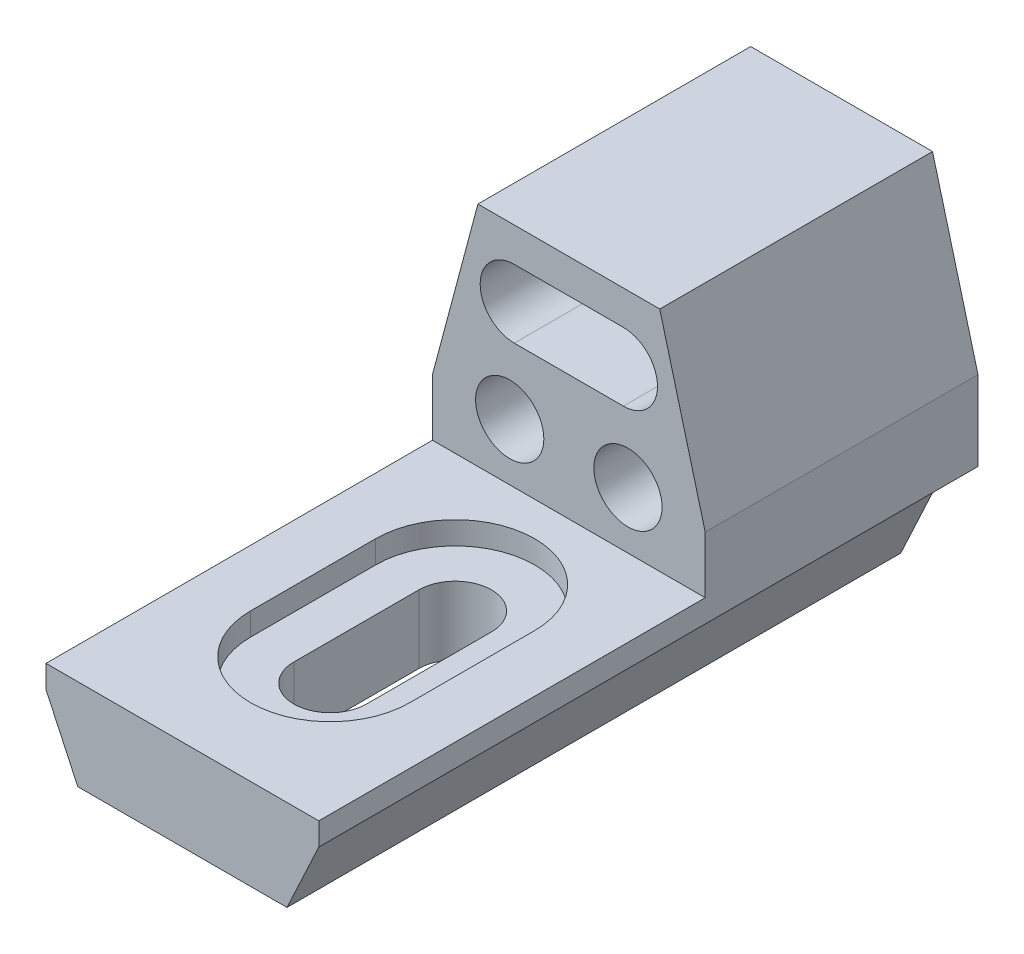
ISO-10303-21;
HEADER;
FILE_DESCRIPTION(('STEP AP214'),'2;1');
FILE_NAME('part.step','',(''),(''),'','','');
FILE_SCHEMA(('AUTOMOTIVE_DESIGN { 1 0 10303 214 1 1 1 1 }'));
ENDSEC;
DATA;
#1=APPLICATION_CONTEXT('core data for automotive mechanical design processes');
#2=APPLICATION_PROTOCOL_DEFINITION('international standard','automotive_design',2000,#1);
#3=PRODUCT_CONTEXT('',#1,'mechanical');
#4=PRODUCT('Part','Part','',(#3));
#5=PRODUCT_RELATED_PRODUCT_CATEGORY('part','',(#4));
#6=PRODUCT_DEFINITION_FORMATION('','',#4);
#7=PRODUCT_DEFINITION_CONTEXT('part definition',#1,'design');
#8=PRODUCT_DEFINITION('design','',#6,#7);
#9=PRODUCT_DEFINITION_SHAPE('','',#8);
#10=(LENGTH_UNIT() NAMED_UNIT(*) SI_UNIT(.MILLI.,.METRE.));
#11=(NAMED_UNIT(*) PLANE_ANGLE_UNIT() SI_UNIT($,.RADIAN.));
#12=(NAMED_UNIT(*) SI_UNIT($,.STERADIAN.) SOLID_ANGLE_UNIT());
#13=UNCERTAINTY_MEASURE_WITH_UNIT(LENGTH_MEASURE(1.E-05),#10,'distance_accuracy_value','');
#14=(GEOMETRIC_REPRESENTATION_CONTEXT(3) GLOBAL_UNCERTAINTY_ASSIGNED_CONTEXT((#13)) GLOBAL_UNIT_ASSIGNED_CONTEXT((#10,
#11,#12)) REPRESENTATION_CONTEXT('',''));
#15=CARTESIAN_POINT('',(0.,0.,0.));
#16=DIRECTION('',(0.,0.,1.));
#17=DIRECTION('',(1.,0.,0.));
#18=AXIS2_PLACEMENT_3D('',#15,#16,#17);
#19=CARTESIAN_POINT('',(0.,30.,50.));
#20=DIRECTION('',(0.,1.,0.));
#21=DIRECTION('',(0.,0.,1.));
#22=AXIS2_PLACEMENT_3D('',#19,#20,#21);
#23=PLANE('',#22);
#24=CARTESIAN_POINT('',(0.,30.,50.));
#25=DIRECTION('',(0.,1.,0.));
#26=DIRECTION('',(0.,0.,1.));
#27=AXIS2_PLACEMENT_3D('',#24,#25,#26);
#28=CIRCLE('',#27,35.);
#29=CARTESIAN_POINT('',(35.,30.,50.));
#30=VERTEX_POINT('',#29);
#31=CARTESIAN_POINT('',(-35.,30.,50.));
#32=VERTEX_POINT('',#31);
#33=EDGE_CURVE('E226',#30,#32,#28,.T.);
#34=ORIENTED_EDGE('',*,*,#33,.T.);
#35=DIRECTION('',(0.,0.,1.));
#36=VECTOR('',#35,1.);
#37=CARTESIAN_POINT('',(-35.,30.,50.));
#38=LINE('',#37,#36);
#39=CARTESIAN_POINT('',(-35.,30.,105.));
#40=VERTEX_POINT('',#39);
#41=EDGE_CURVE('E234',#32,#40,#38,.T.);
#42=ORIENTED_EDGE('',*,*,#41,.T.);
#43=CARTESIAN_POINT('',(0.,30.,105.));
#44=DIRECTION('',(0.,1.,0.));
#45=DIRECTION('',(0.,0.,1.));
#46=AXIS2_PLACEMENT_3D('',#43,#44,#45);
#47=CIRCLE('',#46,35.);
#48=CARTESIAN_POINT('',(35.,30.,105.));
#49=VERTEX_POINT('',#48);
#50=EDGE_CURVE('E240',#40,#49,#47,.T.);
#51=ORIENTED_EDGE('',*,*,#50,.T.);
#52=DIRECTION('',(0.,0.,1.));
#53=VECTOR('',#52,1.);
#54=CARTESIAN_POINT('',(35.,30.,50.));
#55=LINE('',#54,#53);
#56=EDGE_CURVE('E238',#30,#49,#55,.T.);
#57=ORIENTED_EDGE('',*,*,#56,.F.);
#58=EDGE_LOOP('',(#34,#42,#51,#57));
#59=FACE_BOUND('',#58,.T.);
#60=DIRECTION('',(0.,0.,-1.));
#61=VECTOR('',#60,1.);
#62=CARTESIAN_POINT('',(16.,30.,0.));
#63=LINE('',#62,#61);
#64=CARTESIAN_POINT('',(16.,30.,105.));
#65=VERTEX_POINT('',#64);
#66=CARTESIAN_POINT('',(16.,30.,50.));
#67=VERTEX_POINT('',#66);
#68=EDGE_CURVE('E209',#65,#67,#63,.T.);
#69=ORIENTED_EDGE('',*,*,#68,.F.);
#70=CARTESIAN_POINT('',(0.,30.,105.));
#71=DIRECTION('',(0.,1.,0.));
#72=DIRECTION('',(0.,0.,1.));
#73=AXIS2_PLACEMENT_3D('',#70,#71,#72);
#74=CIRCLE('',#73,16.);
#75=CARTESIAN_POINT('',(-16.,30.,105.));
#76=VERTEX_POINT('',#75);
#77=EDGE_CURVE('E200',#65,#76,#74,.F.);
#78=ORIENTED_EDGE('',*,*,#77,.T.);
#79=DIRECTION('',(0.,0.,-1.));
#80=VECTOR('',#79,1.);
#81=CARTESIAN_POINT('',(-16.,30.,0.));
#82=LINE('',#81,#80);
#83=CARTESIAN_POINT('',(-16.,30.,50.));
#84=VERTEX_POINT('',#83);
#85=EDGE_CURVE('E191',#76,#84,#82,.T.);
#86=ORIENTED_EDGE('',*,*,#85,.T.);
#87=CARTESIAN_POINT('',(0.,30.,50.));
#88=DIRECTION('',(0.,1.,0.));
#89=DIRECTION('',(0.,0.,1.));
#90=AXIS2_PLACEMENT_3D('',#87,#88,#89);
#91=CIRCLE('',#90,16.);
#92=EDGE_CURVE('E219',#84,#67,#91,.F.);
#93=ORIENTED_EDGE('',*,*,#92,.T.);
#94=EDGE_LOOP('',(#69,#78,#86,#93));
#95=FACE_BOUND('',#94,.T.);
#96=ADVANCED_FACE('F39',(#59,#95),#23,.T.);
#97=CARTESIAN_POINT('',(-46.0107702553501,0.,-100.));
#98=DIRECTION('',(0.,-1.,0.));
#99=DIRECTION('',(0.,0.,-1.));
#100=AXIS2_PLACEMENT_3D('',#97,#98,#99);
#101=PLANE('',#100);
#102=DIRECTION('',(0.,0.,1.));
#103=VECTOR('',#102,1.);
#104=CARTESIAN_POINT('',(46.0107702553501,0.,-100.));
#105=LINE('',#104,#103);
#106=CARTESIAN_POINT('',(46.0107702553501,0.,-100.));
#107=VERTEX_POINT('',#106);
#108=CARTESIAN_POINT('',(46.0107702553501,0.,170.));
#109=VERTEX_POINT('',#108);
#110=EDGE_CURVE('E390',#107,#109,#105,.T.);
#111=ORIENTED_EDGE('',*,*,#110,.T.);
#112=DIRECTION('',(1.,0.,0.));
#113=VECTOR('',#112,1.);
#114=CARTESIAN_POINT('',(-46.0107702553501,0.,170.));
#115=LINE('',#114,#113);
#116=CARTESIAN_POINT('',(-46.0107702553501,0.,170.));
#117=VERTEX_POINT('',#116);
#118=EDGE_CURVE('E358',#117,#109,#115,.T.);
#119=ORIENTED_EDGE('',*,*,#118,.F.);
#120=DIRECTION('',(0.,0.,1.));
#121=VECTOR('',#120,1.);
#122=CARTESIAN_POINT('',(-46.0107702553501,0.,-100.));
#123=LINE('',#122,#121);
#124=CARTESIAN_POINT('',(-46.0107702553501,0.,-100.));
#125=VERTEX_POINT('',#124);
#126=EDGE_CURVE('E43',#125,#117,#123,.T.);
#127=ORIENTED_EDGE('',*,*,#126,.F.);
#128=DIRECTION('',(1.,0.,0.));
#129=VECTOR('',#128,1.);
#130=CARTESIAN_POINT('',(-46.0107702553501,0.,-100.));
#131=LINE('',#130,#129);
#132=EDGE_CURVE('E380',#125,#107,#131,.T.);
#133=ORIENTED_EDGE('',*,*,#132,.T.);
#134=EDGE_LOOP('',(#111,#119,#127,#133));
#135=FACE_BOUND('',#134,.T.);
#136=CARTESIAN_POINT('',(0.,0.,105.));
#137=DIRECTION('',(0.,-1.,0.));
#138=DIRECTION('',(0.,0.,-1.));
#139=AXIS2_PLACEMENT_3D('',#136,#137,#138);
#140=CIRCLE('',#139,16.);
#141=CARTESIAN_POINT('',(-16.,0.,105.));
#142=VERTEX_POINT('',#141);
#143=CARTESIAN_POINT('',(16.,0.,105.));
#144=VERTEX_POINT('',#143);
#145=EDGE_CURVE('E206',#142,#144,#140,.F.);
#146=ORIENTED_EDGE('',*,*,#145,.T.);
#147=DIRECTION('',(0.,0.,1.));
#148=VECTOR('',#147,1.);
#149=CARTESIAN_POINT('',(16.,0.,0.));
#150=LINE('',#149,#148);
#151=CARTESIAN_POINT('',(16.,0.,50.));
#152=VERTEX_POINT('',#151);
#153=EDGE_CURVE('E220',#152,#144,#150,.T.);
#154=ORIENTED_EDGE('',*,*,#153,.F.);
#155=CARTESIAN_POINT('',(0.,0.,50.));
#156=DIRECTION('',(0.,-1.,0.));
#157=DIRECTION('',(0.,0.,-1.));
#158=AXIS2_PLACEMENT_3D('',#155,#156,#157);
#159=CIRCLE('',#158,16.);
#160=CARTESIAN_POINT('',(-16.,0.,50.));
#161=VERTEX_POINT('',#160);
#162=EDGE_CURVE('E228',#152,#161,#159,.F.);
#163=ORIENTED_EDGE('',*,*,#162,.T.);
#164=DIRECTION('',(0.,0.,1.));
#165=VECTOR('',#164,1.);
#166=CARTESIAN_POINT('',(-16.,0.,0.));
#167=LINE('',#166,#165);
#168=EDGE_CURVE('E215',#161,#142,#167,.T.);
#169=ORIENTED_EDGE('',*,*,#168,.T.);
#170=EDGE_LOOP('',(#146,#154,#163,#169));
#171=FACE_BOUND('',#170,.T.);
#172=ADVANCED_FACE('F395',(#135,#171),#101,.T.);
#173=CARTESIAN_POINT('',(0.,0.,-100.));
#174=DIRECTION('',(0.,0.,1.));
#175=DIRECTION('',(1.,0.,0.));
#176=AXIS2_PLACEMENT_3D('',#173,#174,#175);
#177=PLANE('',#176);
#178=DIRECTION('',(-1.,0.,0.));
#179=VECTOR('',#178,1.);
#180=CARTESIAN_POINT('',(60.,30.,-100.));
#181=LINE('',#180,#179);
#182=CARTESIAN_POINT('',(60.,30.,-100.));
#183=VERTEX_POINT('',#182);
#184=CARTESIAN_POINT('',(-60.,30.,-100.));
#185=VERTEX_POINT('',#184);
#186=EDGE_CURVE('E255',#183,#185,#181,.T.);
#187=ORIENTED_EDGE('',*,*,#186,.F.);
#188=DIRECTION('',(0.422618261740697,0.906307787036651,0.));
#189=VECTOR('',#188,1.);
#190=CARTESIAN_POINT('',(46.0107702553501,0.,-100.));
#191=LINE('',#190,#189);
#192=EDGE_CURVE('E379',#107,#183,#191,.T.);
#193=ORIENTED_EDGE('',*,*,#192,.F.);
#194=ORIENTED_EDGE('',*,*,#132,.F.);
#195=DIRECTION('',(0.422618261740697,-0.906307787036651,0.));
#196=VECTOR('',#195,1.);
#197=CARTESIAN_POINT('',(-60.,30.,-100.));
#198=LINE('',#197,#196);
#199=EDGE_CURVE('E372',#185,#125,#198,.T.);
#200=ORIENTED_EDGE('',*,*,#199,.F.);
#201=EDGE_LOOP('',(#187,#193,#194,#200));
#202=FACE_BOUND('',#201,.T.);
#203=ADVANCED_FACE('F414',(#202),#177,.F.);
#204=CARTESIAN_POINT('',(-60.,30.,-100.));
#205=DIRECTION('',(-0.906307787036651,-0.422618261740697,0.));
#206=DIRECTION('',(0.422618261740697,-0.906307787036651,0.));
#207=AXIS2_PLACEMENT_3D('',#204,#205,#206);
#208=PLANE('',#207);
#209=ORIENTED_EDGE('',*,*,#126,.T.);
#210=DIRECTION('',(0.422618261740697,-0.906307787036651,0.));
#211=VECTOR('',#210,1.);
#212=CARTESIAN_POINT('',(-60.,30.,170.));
#213=LINE('',#212,#211);
#214=CARTESIAN_POINT('',(-60.,30.,170.));
#215=VERTEX_POINT('',#214);
#216=EDGE_CURVE('E353',#215,#117,#213,.T.);
#217=ORIENTED_EDGE('',*,*,#216,.F.);
#218=DIRECTION('',(0.,0.,1.));
#219=VECTOR('',#218,1.);
#220=CARTESIAN_POINT('',(-60.,30.,-100.));
#221=LINE('',#220,#219);
#222=EDGE_CURVE('E11',#185,#215,#221,.T.);
#223=ORIENTED_EDGE('',*,*,#222,.F.);
#224=ORIENTED_EDGE('',*,*,#199,.T.);
#225=EDGE_LOOP('',(#209,#217,#223,#224));
#226=FACE_BOUND('',#225,.T.);
#227=ADVANCED_FACE('F41',(#226),#208,.T.);
#228=CARTESIAN_POINT('',(-60.,40.,-100.));
#229=DIRECTION('',(-1.,0.,0.));
#230=DIRECTION('',(0.,-1.,0.));
#231=AXIS2_PLACEMENT_3D('',#228,#229,#230);
#232=PLANE('',#231);
#233=ORIENTED_EDGE('',*,*,#222,.T.);
#234=DIRECTION('',(0.,-1.,0.));
#235=VECTOR('',#234,1.);
#236=CARTESIAN_POINT('',(-60.,40.,170.));
#237=LINE('',#236,#235);
#238=CARTESIAN_POINT('',(-60.,40.,170.));
#239=VERTEX_POINT('',#238);
#240=EDGE_CURVE('E371',#239,#215,#237,.T.);
#241=ORIENTED_EDGE('',*,*,#240,.F.);
#242=DIRECTION('',(0.,0.,1.));
#243=VECTOR('',#242,1.);
#244=CARTESIAN_POINT('',(-60.,40.,-100.));
#245=LINE('',#244,#243);
#246=CARTESIAN_POINT('',(-60.,40.,0.));
#247=VERTEX_POINT('',#246);
#248=EDGE_CURVE('E48',#247,#239,#245,.T.);
#249=ORIENTED_EDGE('',*,*,#248,.F.);
#250=DIRECTION('',(0.,-1.,0.));
#251=VECTOR('',#250,1.);
#252=CARTESIAN_POINT('',(-60.,40.,0.));
#253=LINE('',#252,#251);
#254=CARTESIAN_POINT('',(-60.,65.,0.));
#255=VERTEX_POINT('',#254);
#256=EDGE_CURVE('E321',#255,#247,#253,.T.);
#257=ORIENTED_EDGE('',*,*,#256,.F.);
#258=DIRECTION('',(0.,0.,1.));
#259=VECTOR('',#258,1.);
#260=CARTESIAN_POINT('',(-60.,65.,-120.));
#261=LINE('',#260,#259);
#262=CARTESIAN_POINT('',(-60.,65.,-120.));
#263=VERTEX_POINT('',#262);
#264=EDGE_CURVE('E349',#263,#255,#261,.T.);
#265=ORIENTED_EDGE('',*,*,#264,.F.);
#266=DIRECTION('',(0.,-1.,0.));
#267=VECTOR('',#266,1.);
#268=CARTESIAN_POINT('',(-60.,40.,-120.));
#269=LINE('',#268,#267);
#270=CARTESIAN_POINT('',(-60.,30.,-120.));
#271=VERTEX_POINT('',#270);
#272=EDGE_CURVE('E329',#263,#271,#269,.T.);
#273=ORIENTED_EDGE('',*,*,#272,.T.);
#274=DIRECTION('',(0.,0.,1.));
#275=VECTOR('',#274,1.);
#276=CARTESIAN_POINT('',(-60.,30.,-120.));
#277=LINE('',#276,#275);
#278=EDGE_CURVE('E262',#271,#185,#277,.T.);
#279=ORIENTED_EDGE('',*,*,#278,.T.);
#280=EDGE_LOOP('',(#233,#241,#249,#257,#265,#273,#279));
#281=FACE_BOUND('',#280,.T.);
#282=ADVANCED_FACE('F401',(#281),#232,.T.);
#283=CARTESIAN_POINT('',(60.,40.,-100.));
#284=DIRECTION('',(0.,1.,0.));
#285=DIRECTION('',(0.,0.,1.));
#286=AXIS2_PLACEMENT_3D('',#283,#284,#285);
#287=PLANE('',#286);
#288=CARTESIAN_POINT('',(0.,40.,50.));
#289=DIRECTION('',(0.,1.,0.));
#290=DIRECTION('',(0.,0.,1.));
#291=AXIS2_PLACEMENT_3D('',#288,#289,#290);
#292=CIRCLE('',#291,35.);
#293=CARTESIAN_POINT('',(35.,40.,50.));
#294=VERTEX_POINT('',#293);
#295=CARTESIAN_POINT('',(-35.,40.,50.));
#296=VERTEX_POINT('',#295);
#297=EDGE_CURVE('E230',#294,#296,#292,.T.);
#298=ORIENTED_EDGE('',*,*,#297,.F.);
#299=DIRECTION('',(0.,0.,1.));
#300=VECTOR('',#299,1.);
#301=CARTESIAN_POINT('',(35.,40.,50.));
#302=LINE('',#301,#300);
#303=CARTESIAN_POINT('',(35.,40.,105.));
#304=VERTEX_POINT('',#303);
#305=EDGE_CURVE('E233',#294,#304,#302,.T.);
#306=ORIENTED_EDGE('',*,*,#305,.T.);
#307=CARTESIAN_POINT('',(0.,40.,105.));
#308=DIRECTION('',(0.,1.,0.));
#309=DIRECTION('',(0.,0.,1.));
#310=AXIS2_PLACEMENT_3D('',#307,#308,#309);
#311=CIRCLE('',#310,35.);
#312=CARTESIAN_POINT('',(-35.,40.,105.));
#313=VERTEX_POINT('',#312);
#314=EDGE_CURVE('E247',#313,#304,#311,.T.);
#315=ORIENTED_EDGE('',*,*,#314,.F.);
#316=DIRECTION('',(0.,0.,1.));
#317=VECTOR('',#316,1.);
#318=CARTESIAN_POINT('',(-35.,40.,50.));
#319=LINE('',#318,#317);
#320=EDGE_CURVE('E245',#296,#313,#319,.T.);
#321=ORIENTED_EDGE('',*,*,#320,.F.);
#322=EDGE_LOOP('',(#298,#306,#315,#321));
#323=FACE_BOUND('',#322,.T.);
#324=DIRECTION('',(1.,0.,0.));
#325=VECTOR('',#324,1.);
#326=CARTESIAN_POINT('',(-60.,40.,0.));
#327=LINE('',#326,#325);
#328=CARTESIAN_POINT('',(60.,40.,0.));
#329=VERTEX_POINT('',#328);
#330=EDGE_CURVE('E309',#247,#329,#327,.T.);
#331=ORIENTED_EDGE('',*,*,#330,.F.);
#332=ORIENTED_EDGE('',*,*,#248,.T.);
#333=DIRECTION('',(-1.,0.,0.));
#334=VECTOR('',#333,1.);
#335=CARTESIAN_POINT('',(60.,40.,170.));
#336=LINE('',#335,#334);
#337=CARTESIAN_POINT('',(60.,40.,170.));
#338=VERTEX_POINT('',#337);
#339=EDGE_CURVE('E366',#338,#239,#336,.T.);
#340=ORIENTED_EDGE('',*,*,#339,.F.);
#341=DIRECTION('',(0.,0.,1.));
#342=VECTOR('',#341,1.);
#343=CARTESIAN_POINT('',(60.,40.,-100.));
#344=LINE('',#343,#342);
#345=EDGE_CURVE('E383',#329,#338,#344,.T.);
#346=ORIENTED_EDGE('',*,*,#345,.F.);
#347=EDGE_LOOP('',(#331,#332,#340,#346));
#348=FACE_BOUND('',#347,.T.);
#349=ADVANCED_FACE('F419',(#323,#348),#287,.T.);
#350=CARTESIAN_POINT('',(60.,30.,-100.));
#351=DIRECTION('',(1.,0.,0.));
#352=DIRECTION('',(0.,1.,0.));
#353=AXIS2_PLACEMENT_3D('',#350,#351,#352);
#354=PLANE('',#353);
#355=DIRECTION('',(0.,0.,1.));
#356=VECTOR('',#355,1.);
#357=CARTESIAN_POINT('',(60.,30.,-100.));
#358=LINE('',#357,#356);
#359=CARTESIAN_POINT('',(60.,30.,170.));
#360=VERTEX_POINT('',#359);
#361=EDGE_CURVE('E387',#183,#360,#358,.T.);
#362=ORIENTED_EDGE('',*,*,#361,.F.);
#363=DIRECTION('',(0.,0.,1.));
#364=VECTOR('',#363,1.);
#365=CARTESIAN_POINT('',(60.,30.,-120.));
#366=LINE('',#365,#364);
#367=CARTESIAN_POINT('',(60.,30.,-120.));
#368=VERTEX_POINT('',#367);
#369=EDGE_CURVE('E267',#368,#183,#366,.T.);
#370=ORIENTED_EDGE('',*,*,#369,.F.);
#371=DIRECTION('',(0.,1.,0.));
#372=VECTOR('',#371,1.);
#373=CARTESIAN_POINT('',(60.,65.,-120.));
#374=LINE('',#373,#372);
#375=CARTESIAN_POINT('',(60.,65.,-120.));
#376=VERTEX_POINT('',#375);
#377=EDGE_CURVE('E320',#368,#376,#374,.T.);
#378=ORIENTED_EDGE('',*,*,#377,.T.);
#379=DIRECTION('',(0.,0.,1.));
#380=VECTOR('',#379,1.);
#381=CARTESIAN_POINT('',(60.,65.,-120.));
#382=LINE('',#381,#380);
#383=CARTESIAN_POINT('',(60.,65.,0.));
#384=VERTEX_POINT('',#383);
#385=EDGE_CURVE('E335',#376,#384,#382,.T.);
#386=ORIENTED_EDGE('',*,*,#385,.T.);
#387=DIRECTION('',(0.,1.,0.));
#388=VECTOR('',#387,1.);
#389=CARTESIAN_POINT('',(60.,65.,0.));
#390=LINE('',#389,#388);
#391=EDGE_CURVE('E333',#329,#384,#390,.T.);
#392=ORIENTED_EDGE('',*,*,#391,.F.);
#393=ORIENTED_EDGE('',*,*,#345,.T.);
#394=DIRECTION('',(0.,1.,0.));
#395=VECTOR('',#394,1.);
#396=CARTESIAN_POINT('',(60.,30.,170.));
#397=LINE('',#396,#395);
#398=EDGE_CURVE('E364',#360,#338,#397,.T.);
#399=ORIENTED_EDGE('',*,*,#398,.F.);
#400=EDGE_LOOP('',(#362,#370,#378,#386,#392,#393,#399));
#401=FACE_BOUND('',#400,.T.);
#402=ADVANCED_FACE('F418',(#401),#354,.T.);
#403=CARTESIAN_POINT('',(46.0107702553501,0.,-100.));
#404=DIRECTION('',(0.906307787036651,-0.422618261740697,0.));
#405=DIRECTION('',(0.422618261740697,0.906307787036651,0.));
#406=AXIS2_PLACEMENT_3D('',#403,#404,#405);
#407=PLANE('',#406);
#408=ORIENTED_EDGE('',*,*,#361,.T.);
#409=DIRECTION('',(0.422618261740697,0.906307787036651,0.));
#410=VECTOR('',#409,1.);
#411=CARTESIAN_POINT('',(46.0107702553501,0.,170.));
#412=LINE('',#411,#410);
#413=EDGE_CURVE('E362',#109,#360,#412,.T.);
#414=ORIENTED_EDGE('',*,*,#413,.F.);
#415=ORIENTED_EDGE('',*,*,#110,.F.);
#416=ORIENTED_EDGE('',*,*,#192,.T.);
#417=EDGE_LOOP('',(#408,#414,#415,#416));
#418=FACE_BOUND('',#417,.T.);
#419=ADVANCED_FACE('F416',(#418),#407,.T.);
#420=CARTESIAN_POINT('',(0.,0.,170.));
#421=DIRECTION('',(0.,0.,1.));
#422=DIRECTION('',(1.,0.,0.));
#423=AXIS2_PLACEMENT_3D('',#420,#421,#422);
#424=PLANE('',#423);
#425=ORIENTED_EDGE('',*,*,#216,.T.);
#426=ORIENTED_EDGE('',*,*,#118,.T.);
#427=ORIENTED_EDGE('',*,*,#413,.T.);
#428=ORIENTED_EDGE('',*,*,#398,.T.);
#429=ORIENTED_EDGE('',*,*,#339,.T.);
#430=ORIENTED_EDGE('',*,*,#240,.T.);
#431=EDGE_LOOP('',(#425,#426,#427,#428,#429,#430));
#432=FACE_BOUND('',#431,.T.);
#433=ADVANCED_FACE('F399',(#432),#424,.T.);
#434=CARTESIAN_POINT('',(-60.,65.,-120.));
#435=DIRECTION('',(-0.966234939601246,0.257662650560332,0.));
#436=DIRECTION('',(-0.257662650560332,-0.966234939601246,0.));
#437=AXIS2_PLACEMENT_3D('',#434,#435,#436);
#438=PLANE('',#437);
#439=DIRECTION('',(-0.257662650560332,-0.966234939601246,0.));
#440=VECTOR('',#439,1.);
#441=CARTESIAN_POINT('',(-60.,65.,0.));
#442=LINE('',#441,#440);
#443=CARTESIAN_POINT('',(-40.,140.,0.));
#444=VERTEX_POINT('',#443);
#445=EDGE_CURVE('E343',#444,#255,#442,.T.);
#446=ORIENTED_EDGE('',*,*,#445,.F.);
#447=DIRECTION('',(0.,0.,1.));
#448=VECTOR('',#447,1.);
#449=CARTESIAN_POINT('',(-40.,140.,-120.));
#450=LINE('',#449,#448);
#451=CARTESIAN_POINT('',(-40.,140.,-120.));
#452=VERTEX_POINT('',#451);
#453=EDGE_CURVE('E354',#452,#444,#450,.T.);
#454=ORIENTED_EDGE('',*,*,#453,.F.);
#455=DIRECTION('',(-0.257662650560332,-0.966234939601246,0.));
#456=VECTOR('',#455,1.);
#457=CARTESIAN_POINT('',(-60.,65.,-120.));
#458=LINE('',#457,#456);
#459=EDGE_CURVE('E330',#452,#263,#458,.T.);
#460=ORIENTED_EDGE('',*,*,#459,.T.);
#461=ORIENTED_EDGE('',*,*,#264,.T.);
#462=EDGE_LOOP('',(#446,#454,#460,#461));
#463=FACE_BOUND('',#462,.T.);
#464=ADVANCED_FACE('F428',(#463),#438,.T.);
#465=CARTESIAN_POINT('',(-40.,140.,-120.));
#466=DIRECTION('',(0.,1.,0.));
#467=DIRECTION('',(0.,0.,1.));
#468=AXIS2_PLACEMENT_3D('',#465,#466,#467);
#469=PLANE('',#468);
#470=DIRECTION('',(-1.,0.,0.));
#471=VECTOR('',#470,1.);
#472=CARTESIAN_POINT('',(-40.,140.,0.));
#473=LINE('',#472,#471);
#474=CARTESIAN_POINT('',(40.,140.,0.));
#475=VERTEX_POINT('',#474);
#476=EDGE_CURVE('E341',#475,#444,#473,.T.);
#477=ORIENTED_EDGE('',*,*,#476,.F.);
#478=DIRECTION('',(0.,0.,1.));
#479=VECTOR('',#478,1.);
#480=CARTESIAN_POINT('',(40.,140.,-120.));
#481=LINE('',#480,#479);
#482=CARTESIAN_POINT('',(40.,140.,-120.));
#483=VERTEX_POINT('',#482);
#484=EDGE_CURVE('E355',#483,#475,#481,.T.);
#485=ORIENTED_EDGE('',*,*,#484,.F.);
#486=DIRECTION('',(-1.,0.,0.));
#487=VECTOR('',#486,1.);
#488=CARTESIAN_POINT('',(-40.,140.,-120.));
#489=LINE('',#488,#487);
#490=EDGE_CURVE('E322',#483,#452,#489,.T.);
#491=ORIENTED_EDGE('',*,*,#490,.T.);
#492=ORIENTED_EDGE('',*,*,#453,.T.);
#493=EDGE_LOOP('',(#477,#485,#491,#492));
#494=FACE_BOUND('',#493,.T.);
#495=ADVANCED_FACE('F437',(#494),#469,.T.);
#496=CARTESIAN_POINT('',(40.,140.,-120.));
#497=DIRECTION('',(0.966234939601246,0.257662650560332,0.));
#498=DIRECTION('',(-0.257662650560332,0.966234939601246,0.));
#499=AXIS2_PLACEMENT_3D('',#496,#497,#498);
#500=PLANE('',#499);
#501=DIRECTION('',(-0.257662650560332,0.966234939601246,0.));
#502=VECTOR('',#501,1.);
#503=CARTESIAN_POINT('',(40.,140.,0.));
#504=LINE('',#503,#502);
#505=EDGE_CURVE('E337',#384,#475,#504,.T.);
#506=ORIENTED_EDGE('',*,*,#505,.F.);
#507=ORIENTED_EDGE('',*,*,#385,.F.);
#508=DIRECTION('',(-0.257662650560332,0.966234939601246,0.));
#509=VECTOR('',#508,1.);
#510=CARTESIAN_POINT('',(40.,140.,-120.));
#511=LINE('',#510,#509);
#512=EDGE_CURVE('E319',#376,#483,#511,.T.);
#513=ORIENTED_EDGE('',*,*,#512,.T.);
#514=ORIENTED_EDGE('',*,*,#484,.T.);
#515=EDGE_LOOP('',(#506,#507,#513,#514));
#516=FACE_BOUND('',#515,.T.);
#517=ADVANCED_FACE('F434',(#516),#500,.T.);
#518=CARTESIAN_POINT('',(0.,0.,-120.));
#519=DIRECTION('',(0.,0.,-1.));
#520=DIRECTION('',(-1.,0.,0.));
#521=AXIS2_PLACEMENT_3D('',#518,#519,#520);
#522=PLANE('',#521);
#523=CARTESIAN_POINT('',(26.,65.,-120.));
#524=DIRECTION('',(0.,0.,1.));
#525=DIRECTION('',(1.,0.,0.));
#526=AXIS2_PLACEMENT_3D('',#523,#524,#525);
#527=CIRCLE('',#526,15.);
#528=CARTESIAN_POINT('',(41.,65.,-120.));
#529=VERTEX_POINT('',#528);
#530=EDGE_CURVE('E272',#529,#529,#527,.T.);
#531=ORIENTED_EDGE('',*,*,#530,.T.);
#532=EDGE_LOOP('',(#531));
#533=FACE_BOUND('',#532,.T.);
#534=CARTESIAN_POINT('',(-26.,65.,-120.));
#535=DIRECTION('',(0.,0.,1.));
#536=DIRECTION('',(1.,0.,0.));
#537=AXIS2_PLACEMENT_3D('',#534,#535,#536);
#538=CIRCLE('',#537,15.);
#539=CARTESIAN_POINT('',(-11.,65.,-120.));
#540=VERTEX_POINT('',#539);
#541=EDGE_CURVE('E276',#540,#540,#538,.T.);
#542=ORIENTED_EDGE('',*,*,#541,.T.);
#543=EDGE_LOOP('',(#542));
#544=FACE_BOUND('',#543,.T.);
#545=CARTESIAN_POINT('',(-24.,110.,-120.));
#546=DIRECTION('',(0.,0.,1.));
#547=DIRECTION('',(1.,0.,0.));
#548=AXIS2_PLACEMENT_3D('',#545,#546,#547);
#549=CIRCLE('',#548,15.);
#550=CARTESIAN_POINT('',(-24.,125.,-120.));
#551=VERTEX_POINT('',#550);
#552=CARTESIAN_POINT('',(-24.,95.,-120.));
#553=VERTEX_POINT('',#552);
#554=EDGE_CURVE('E281',#551,#553,#549,.T.);
#555=ORIENTED_EDGE('',*,*,#554,.T.);
#556=DIRECTION('',(1.,0.,0.));
#557=VECTOR('',#556,1.);
#558=CARTESIAN_POINT('',(-24.,95.,-120.));
#559=LINE('',#558,#557);
#560=CARTESIAN_POINT('',(24.,95.,-120.));
#561=VERTEX_POINT('',#560);
#562=EDGE_CURVE('E289',#553,#561,#559,.T.);
#563=ORIENTED_EDGE('',*,*,#562,.T.);
#564=CARTESIAN_POINT('',(24.,110.,-120.));
#565=DIRECTION('',(0.,0.,1.));
#566=DIRECTION('',(1.,0.,0.));
#567=AXIS2_PLACEMENT_3D('',#564,#565,#566);
#568=CIRCLE('',#567,15.);
#569=CARTESIAN_POINT('',(24.,125.,-120.));
#570=VERTEX_POINT('',#569);
#571=EDGE_CURVE('E295',#561,#570,#568,.T.);
#572=ORIENTED_EDGE('',*,*,#571,.T.);
#573=DIRECTION('',(-1.,0.,0.));
#574=VECTOR('',#573,1.);
#575=CARTESIAN_POINT('',(-24.,125.,-120.));
#576=LINE('',#575,#574);
#577=EDGE_CURVE('E293',#570,#551,#576,.T.);
#578=ORIENTED_EDGE('',*,*,#577,.T.);
#579=EDGE_LOOP('',(#555,#563,#572,#578));
#580=FACE_BOUND('',#579,.T.);
#581=ORIENTED_EDGE('',*,*,#377,.F.);
#582=DIRECTION('',(-1.,0.,0.));
#583=VECTOR('',#582,1.);
#584=CARTESIAN_POINT('',(60.,30.,-120.));
#585=LINE('',#584,#583);
#586=EDGE_CURVE('E261',#368,#271,#585,.T.);
#587=ORIENTED_EDGE('',*,*,#586,.T.);
#588=ORIENTED_EDGE('',*,*,#272,.F.);
#589=ORIENTED_EDGE('',*,*,#459,.F.);
#590=ORIENTED_EDGE('',*,*,#490,.F.);
#591=ORIENTED_EDGE('',*,*,#512,.F.);
#592=EDGE_LOOP('',(#581,#587,#588,#589,#590,#591));
#593=FACE_BOUND('',#592,.T.);
#594=ADVANCED_FACE('F431',(#533,#544,#580,#593),#522,.T.);
#595=CARTESIAN_POINT('',(0.,0.,0.));
#596=DIRECTION('',(0.,0.,-1.));
#597=DIRECTION('',(-1.,0.,0.));
#598=AXIS2_PLACEMENT_3D('',#595,#596,#597);
#599=PLANE('',#598);
#600=CARTESIAN_POINT('',(26.,65.,0.));
#601=DIRECTION('',(0.,0.,1.));
#602=DIRECTION('',(1.,0.,0.));
#603=AXIS2_PLACEMENT_3D('',#600,#601,#602);
#604=CIRCLE('',#603,15.);
#605=CARTESIAN_POINT('',(41.,65.,0.));
#606=VERTEX_POINT('',#605);
#607=EDGE_CURVE('E275',#606,#606,#604,.T.);
#608=ORIENTED_EDGE('',*,*,#607,.F.);
#609=EDGE_LOOP('',(#608));
#610=FACE_BOUND('',#609,.T.);
#611=CARTESIAN_POINT('',(-26.,65.,0.));
#612=DIRECTION('',(0.,0.,1.));
#613=DIRECTION('',(1.,0.,0.));
#614=AXIS2_PLACEMENT_3D('',#611,#612,#613);
#615=CIRCLE('',#614,15.);
#616=CARTESIAN_POINT('',(-11.,65.,0.));
#617=VERTEX_POINT('',#616);
#618=EDGE_CURVE('E277',#617,#617,#615,.T.);
#619=ORIENTED_EDGE('',*,*,#618,.F.);
#620=EDGE_LOOP('',(#619));
#621=FACE_BOUND('',#620,.T.);
#622=DIRECTION('',(1.,0.,0.));
#623=VECTOR('',#622,1.);
#624=CARTESIAN_POINT('',(-24.,95.,0.));
#625=LINE('',#624,#623);
#626=CARTESIAN_POINT('',(-24.,95.,0.));
#627=VERTEX_POINT('',#626);
#628=CARTESIAN_POINT('',(24.,95.,0.));
#629=VERTEX_POINT('',#628);
#630=EDGE_CURVE('E296',#627,#629,#625,.T.);
#631=ORIENTED_EDGE('',*,*,#630,.F.);
#632=CARTESIAN_POINT('',(-24.,110.,0.));
#633=DIRECTION('',(0.,0.,1.));
#634=DIRECTION('',(1.,0.,0.));
#635=AXIS2_PLACEMENT_3D('',#632,#633,#634);
#636=CIRCLE('',#635,15.);
#637=CARTESIAN_POINT('',(-24.,125.,0.));
#638=VERTEX_POINT('',#637);
#639=EDGE_CURVE('E284',#638,#627,#636,.T.);
#640=ORIENTED_EDGE('',*,*,#639,.F.);
#641=DIRECTION('',(-1.,0.,0.));
#642=VECTOR('',#641,1.);
#643=CARTESIAN_POINT('',(-24.,125.,0.));
#644=LINE('',#643,#642);
#645=CARTESIAN_POINT('',(24.,125.,0.));
#646=VERTEX_POINT('',#645);
#647=EDGE_CURVE('E288',#646,#638,#644,.T.);
#648=ORIENTED_EDGE('',*,*,#647,.F.);
#649=CARTESIAN_POINT('',(24.,110.,0.));
#650=DIRECTION('',(0.,0.,1.));
#651=DIRECTION('',(1.,0.,0.));
#652=AXIS2_PLACEMENT_3D('',#649,#650,#651);
#653=CIRCLE('',#652,15.);
#654=EDGE_CURVE('E304',#629,#646,#653,.T.);
#655=ORIENTED_EDGE('',*,*,#654,.F.);
#656=EDGE_LOOP('',(#631,#640,#648,#655));
#657=FACE_BOUND('',#656,.T.);
#658=ORIENTED_EDGE('',*,*,#330,.T.);
#659=ORIENTED_EDGE('',*,*,#391,.T.);
#660=ORIENTED_EDGE('',*,*,#505,.T.);
#661=ORIENTED_EDGE('',*,*,#476,.T.);
#662=ORIENTED_EDGE('',*,*,#445,.T.);
#663=ORIENTED_EDGE('',*,*,#256,.T.);
#664=EDGE_LOOP('',(#658,#659,#660,#661,#662,#663));
#665=FACE_BOUND('',#664,.T.);
#666=ADVANCED_FACE('F421',(#610,#621,#657,#665),#599,.F.);
#667=CARTESIAN_POINT('',(-24.,110.,-120.));
#668=DIRECTION('',(0.,0.,1.));
#669=DIRECTION('',(1.,0.,0.));
#670=AXIS2_PLACEMENT_3D('',#667,#668,#669);
#671=CYLINDRICAL_SURFACE('',#670,15.);
#672=ORIENTED_EDGE('',*,*,#639,.T.);
#673=DIRECTION('',(0.,0.,1.));
#674=VECTOR('',#673,1.);
#675=CARTESIAN_POINT('',(-24.,95.,-120.));
#676=LINE('',#675,#674);
#677=EDGE_CURVE('E297',#553,#627,#676,.T.);
#678=ORIENTED_EDGE('',*,*,#677,.F.);
#679=ORIENTED_EDGE('',*,*,#554,.F.);
#680=DIRECTION('',(0.,0.,1.));
#681=VECTOR('',#680,1.);
#682=CARTESIAN_POINT('',(-24.,125.,-120.));
#683=LINE('',#682,#681);
#684=EDGE_CURVE('E306',#551,#638,#683,.T.);
#685=ORIENTED_EDGE('',*,*,#684,.T.);
#686=EDGE_LOOP('',(#672,#678,#679,#685));
#687=FACE_BOUND('',#686,.T.);
#688=ADVANCED_FACE('F488',(#687),#671,.F.);
#689=CARTESIAN_POINT('',(-24.,125.,-120.));
#690=DIRECTION('',(0.,1.,0.));
#691=DIRECTION('',(0.,0.,1.));
#692=AXIS2_PLACEMENT_3D('',#689,#690,#691);
#693=PLANE('',#692);
#694=ORIENTED_EDGE('',*,*,#647,.T.);
#695=ORIENTED_EDGE('',*,*,#684,.F.);
#696=ORIENTED_EDGE('',*,*,#577,.F.);
#697=DIRECTION('',(0.,0.,1.));
#698=VECTOR('',#697,1.);
#699=CARTESIAN_POINT('',(24.,125.,-120.));
#700=LINE('',#699,#698);
#701=EDGE_CURVE('E313',#570,#646,#700,.T.);
#702=ORIENTED_EDGE('',*,*,#701,.T.);
#703=EDGE_LOOP('',(#694,#695,#696,#702));
#704=FACE_BOUND('',#703,.T.);
#705=ADVANCED_FACE('F482',(#704),#693,.F.);
#706=CARTESIAN_POINT('',(24.,110.,-120.));
#707=DIRECTION('',(0.,0.,1.));
#708=DIRECTION('',(1.,0.,0.));
#709=AXIS2_PLACEMENT_3D('',#706,#707,#708);
#710=CYLINDRICAL_SURFACE('',#709,15.);
#711=ORIENTED_EDGE('',*,*,#654,.T.);
#712=ORIENTED_EDGE('',*,*,#701,.F.);
#713=ORIENTED_EDGE('',*,*,#571,.F.);
#714=DIRECTION('',(0.,0.,1.));
#715=VECTOR('',#714,1.);
#716=CARTESIAN_POINT('',(24.,95.,-120.));
#717=LINE('',#716,#715);
#718=EDGE_CURVE('E311',#561,#629,#717,.T.);
#719=ORIENTED_EDGE('',*,*,#718,.T.);
#720=EDGE_LOOP('',(#711,#712,#713,#719));
#721=FACE_BOUND('',#720,.T.);
#722=ADVANCED_FACE('F490',(#721),#710,.F.);
#723=CARTESIAN_POINT('',(-24.,95.,-120.));
#724=DIRECTION('',(0.,-1.,0.));
#725=DIRECTION('',(0.,0.,-1.));
#726=AXIS2_PLACEMENT_3D('',#723,#724,#725);
#727=PLANE('',#726);
#728=ORIENTED_EDGE('',*,*,#630,.T.);
#729=ORIENTED_EDGE('',*,*,#718,.F.);
#730=ORIENTED_EDGE('',*,*,#562,.F.);
#731=ORIENTED_EDGE('',*,*,#677,.T.);
#732=EDGE_LOOP('',(#728,#729,#730,#731));
#733=FACE_BOUND('',#732,.T.);
#734=ADVANCED_FACE('F485',(#733),#727,.F.);
#735=CARTESIAN_POINT('',(-26.,65.,-120.));
#736=DIRECTION('',(0.,0.,1.));
#737=DIRECTION('',(1.,0.,0.));
#738=AXIS2_PLACEMENT_3D('',#735,#736,#737);
#739=CYLINDRICAL_SURFACE('',#738,15.);
#740=ORIENTED_EDGE('',*,*,#541,.F.);
#741=EDGE_LOOP('',(#740));
#742=FACE_BOUND('',#741,.T.);
#743=ORIENTED_EDGE('',*,*,#618,.T.);
#744=EDGE_LOOP('',(#743));
#745=FACE_BOUND('',#744,.T.);
#746=ADVANCED_FACE('F476',(#742,#745),#739,.F.);
#747=CARTESIAN_POINT('',(26.,65.,-120.));
#748=DIRECTION('',(0.,0.,1.));
#749=DIRECTION('',(1.,0.,0.));
#750=AXIS2_PLACEMENT_3D('',#747,#748,#749);
#751=CYLINDRICAL_SURFACE('',#750,15.);
#752=ORIENTED_EDGE('',*,*,#530,.F.);
#753=EDGE_LOOP('',(#752));
#754=FACE_BOUND('',#753,.T.);
#755=ORIENTED_EDGE('',*,*,#607,.T.);
#756=EDGE_LOOP('',(#755));
#757=FACE_BOUND('',#756,.T.);
#758=ADVANCED_FACE('F474',(#754,#757),#751,.F.);
#759=CARTESIAN_POINT('',(60.,30.,-120.));
#760=DIRECTION('',(0.,1.,0.));
#761=DIRECTION('',(0.,0.,1.));
#762=AXIS2_PLACEMENT_3D('',#759,#760,#761);
#763=PLANE('',#762);
#764=ORIENTED_EDGE('',*,*,#186,.T.);
#765=ORIENTED_EDGE('',*,*,#278,.F.);
#766=ORIENTED_EDGE('',*,*,#586,.F.);
#767=ORIENTED_EDGE('',*,*,#369,.T.);
#768=EDGE_LOOP('',(#764,#765,#766,#767));
#769=FACE_BOUND('',#768,.T.);
#770=ADVANCED_FACE('F409',(#769),#763,.F.);
#771=CARTESIAN_POINT('',(0.,30.,50.));
#772=DIRECTION('',(0.,1.,0.));
#773=DIRECTION('',(0.,0.,1.));
#774=AXIS2_PLACEMENT_3D('',#771,#772,#773);
#775=CYLINDRICAL_SURFACE('',#774,35.);
#776=ORIENTED_EDGE('',*,*,#297,.T.);
#777=DIRECTION('',(0.,1.,0.));
#778=VECTOR('',#777,1.);
#779=CARTESIAN_POINT('',(-35.,30.,50.));
#780=LINE('',#779,#778);
#781=EDGE_CURVE('E244',#32,#296,#780,.T.);
#782=ORIENTED_EDGE('',*,*,#781,.F.);
#783=ORIENTED_EDGE('',*,*,#33,.F.);
#784=DIRECTION('',(0.,1.,0.));
#785=VECTOR('',#784,1.);
#786=CARTESIAN_POINT('',(35.,30.,50.));
#787=LINE('',#786,#785);
#788=EDGE_CURVE('E252',#30,#294,#787,.T.);
#789=ORIENTED_EDGE('',*,*,#788,.T.);
#790=EDGE_LOOP('',(#776,#782,#783,#789));
#791=FACE_BOUND('',#790,.T.);
#792=ADVANCED_FACE('F464',(#791),#775,.F.);
#793=CARTESIAN_POINT('',(35.,30.,50.));
#794=DIRECTION('',(-1.,0.,0.));
#795=DIRECTION('',(0.,0.,1.));
#796=AXIS2_PLACEMENT_3D('',#793,#794,#795);
#797=PLANE('',#796);
#798=ORIENTED_EDGE('',*,*,#305,.F.);
#799=ORIENTED_EDGE('',*,*,#788,.F.);
#800=ORIENTED_EDGE('',*,*,#56,.T.);
#801=DIRECTION('',(0.,1.,0.));
#802=VECTOR('',#801,1.);
#803=CARTESIAN_POINT('',(35.,30.,105.));
#804=LINE('',#803,#802);
#805=EDGE_CURVE('E254',#49,#304,#804,.T.);
#806=ORIENTED_EDGE('',*,*,#805,.T.);
#807=EDGE_LOOP('',(#798,#799,#800,#806));
#808=FACE_BOUND('',#807,.T.);
#809=ADVANCED_FACE('F456',(#808),#797,.T.);
#810=CARTESIAN_POINT('',(0.,30.,105.));
#811=DIRECTION('',(0.,1.,0.));
#812=DIRECTION('',(0.,0.,1.));
#813=AXIS2_PLACEMENT_3D('',#810,#811,#812);
#814=CYLINDRICAL_SURFACE('',#813,35.);
#815=ORIENTED_EDGE('',*,*,#314,.T.);
#816=ORIENTED_EDGE('',*,*,#805,.F.);
#817=ORIENTED_EDGE('',*,*,#50,.F.);
#818=DIRECTION('',(0.,1.,0.));
#819=VECTOR('',#818,1.);
#820=CARTESIAN_POINT('',(-35.,30.,105.));
#821=LINE('',#820,#819);
#822=EDGE_CURVE('E260',#40,#313,#821,.T.);
#823=ORIENTED_EDGE('',*,*,#822,.T.);
#824=EDGE_LOOP('',(#815,#816,#817,#823));
#825=FACE_BOUND('',#824,.T.);
#826=ADVANCED_FACE('F463',(#825),#814,.F.);
#827=CARTESIAN_POINT('',(-35.,30.,50.));
#828=DIRECTION('',(-1.,0.,0.));
#829=DIRECTION('',(0.,0.,1.));
#830=AXIS2_PLACEMENT_3D('',#827,#828,#829);
#831=PLANE('',#830);
#832=ORIENTED_EDGE('',*,*,#320,.T.);
#833=ORIENTED_EDGE('',*,*,#822,.F.);
#834=ORIENTED_EDGE('',*,*,#41,.F.);
#835=ORIENTED_EDGE('',*,*,#781,.T.);
#836=EDGE_LOOP('',(#832,#833,#834,#835));
#837=FACE_BOUND('',#836,.T.);
#838=ADVANCED_FACE('F466',(#837),#831,.F.);
#839=CARTESIAN_POINT('',(16.,-0.001000000000001,0.));
#840=DIRECTION('',(-1.,0.,0.));
#841=DIRECTION('',(0.,0.,1.));
#842=AXIS2_PLACEMENT_3D('',#839,#840,#841);
#843=PLANE('',#842);
#844=ORIENTED_EDGE('',*,*,#153,.T.);
#845=DIRECTION('',(0.,1.,0.));
#846=VECTOR('',#845,1.);
#847=CARTESIAN_POINT('',(16.,-0.001000000000001,105.));
#848=LINE('',#847,#846);
#849=EDGE_CURVE('E210',#144,#65,#848,.T.);
#850=ORIENTED_EDGE('',*,*,#849,.T.);
#851=ORIENTED_EDGE('',*,*,#68,.T.);
#852=DIRECTION('',(0.,1.,0.));
#853=VECTOR('',#852,1.);
#854=CARTESIAN_POINT('',(16.,-0.001000000000001,50.));
#855=LINE('',#854,#853);
#856=EDGE_CURVE('E218',#152,#67,#855,.T.);
#857=ORIENTED_EDGE('',*,*,#856,.F.);
#858=EDGE_LOOP('',(#844,#850,#851,#857));
#859=FACE_BOUND('',#858,.T.);
#860=ADVANCED_FACE('F457',(#859),#843,.T.);
#861=CARTESIAN_POINT('',(0.,-0.001000000000001,105.));
#862=DIRECTION('',(0.,1.,0.));
#863=DIRECTION('',(0.,0.,1.));
#864=AXIS2_PLACEMENT_3D('',#861,#862,#863);
#865=CYLINDRICAL_SURFACE('',#864,16.);
#866=DIRECTION('',(0.,1.,0.));
#867=VECTOR('',#866,1.);
#868=CARTESIAN_POINT('',(-16.,-0.001000000000001,105.));
#869=LINE('',#868,#867);
#870=EDGE_CURVE('E193',#142,#76,#869,.T.);
#871=ORIENTED_EDGE('',*,*,#870,.T.);
#872=ORIENTED_EDGE('',*,*,#77,.F.);
#873=ORIENTED_EDGE('',*,*,#849,.F.);
#874=ORIENTED_EDGE('',*,*,#145,.F.);
#875=EDGE_LOOP('',(#871,#872,#873,#874));
#876=FACE_BOUND('',#875,.T.);
#877=ADVANCED_FACE('F205',(#876),#865,.F.);
#878=CARTESIAN_POINT('',(-16.,-0.001000000000001,0.));
#879=DIRECTION('',(-1.,0.,0.));
#880=DIRECTION('',(0.,0.,1.));
#881=AXIS2_PLACEMENT_3D('',#878,#879,#880);
#882=PLANE('',#881);
#883=DIRECTION('',(0.,1.,0.));
#884=VECTOR('',#883,1.);
#885=CARTESIAN_POINT('',(-16.,-0.001000000000001,50.));
#886=LINE('',#885,#884);
#887=EDGE_CURVE('E57',#161,#84,#886,.T.);
#888=ORIENTED_EDGE('',*,*,#887,.T.);
#889=ORIENTED_EDGE('',*,*,#85,.F.);
#890=ORIENTED_EDGE('',*,*,#870,.F.);
#891=ORIENTED_EDGE('',*,*,#168,.F.);
#892=EDGE_LOOP('',(#888,#889,#890,#891));
#893=FACE_BOUND('',#892,.T.);
#894=ADVANCED_FACE('F194',(#893),#882,.F.);
#895=CARTESIAN_POINT('',(0.,-0.001000000000001,50.));
#896=DIRECTION('',(0.,1.,0.));
#897=DIRECTION('',(0.,0.,1.));
#898=AXIS2_PLACEMENT_3D('',#895,#896,#897);
#899=CYLINDRICAL_SURFACE('',#898,16.);
#900=ORIENTED_EDGE('',*,*,#856,.T.);
#901=ORIENTED_EDGE('',*,*,#92,.F.);
#902=ORIENTED_EDGE('',*,*,#887,.F.);
#903=ORIENTED_EDGE('',*,*,#162,.F.);
#904=EDGE_LOOP('',(#900,#901,#902,#903));
#905=FACE_BOUND('',#904,.T.);
#906=ADVANCED_FACE('F656',(#905),#899,.F.);
#907=CLOSED_SHELL('',(#96,#172,#203,#227,#282,#349,#402,#419,#433,#464,#495,#517,#594,#666,#688,
#705,#722,#734,#746,#758,#770,#792,#809,#826,#838,#860,#877,#894,#906));
#908=MANIFOLD_SOLID_BREP('B2',#907);
#909=ADVANCED_BREP_SHAPE_REPRESENTATION('',(#18,#908),#14);
#910=SHAPE_DEFINITION_REPRESENTATION(#9,#909);
ENDSEC;
END-ISO-10303-21;
